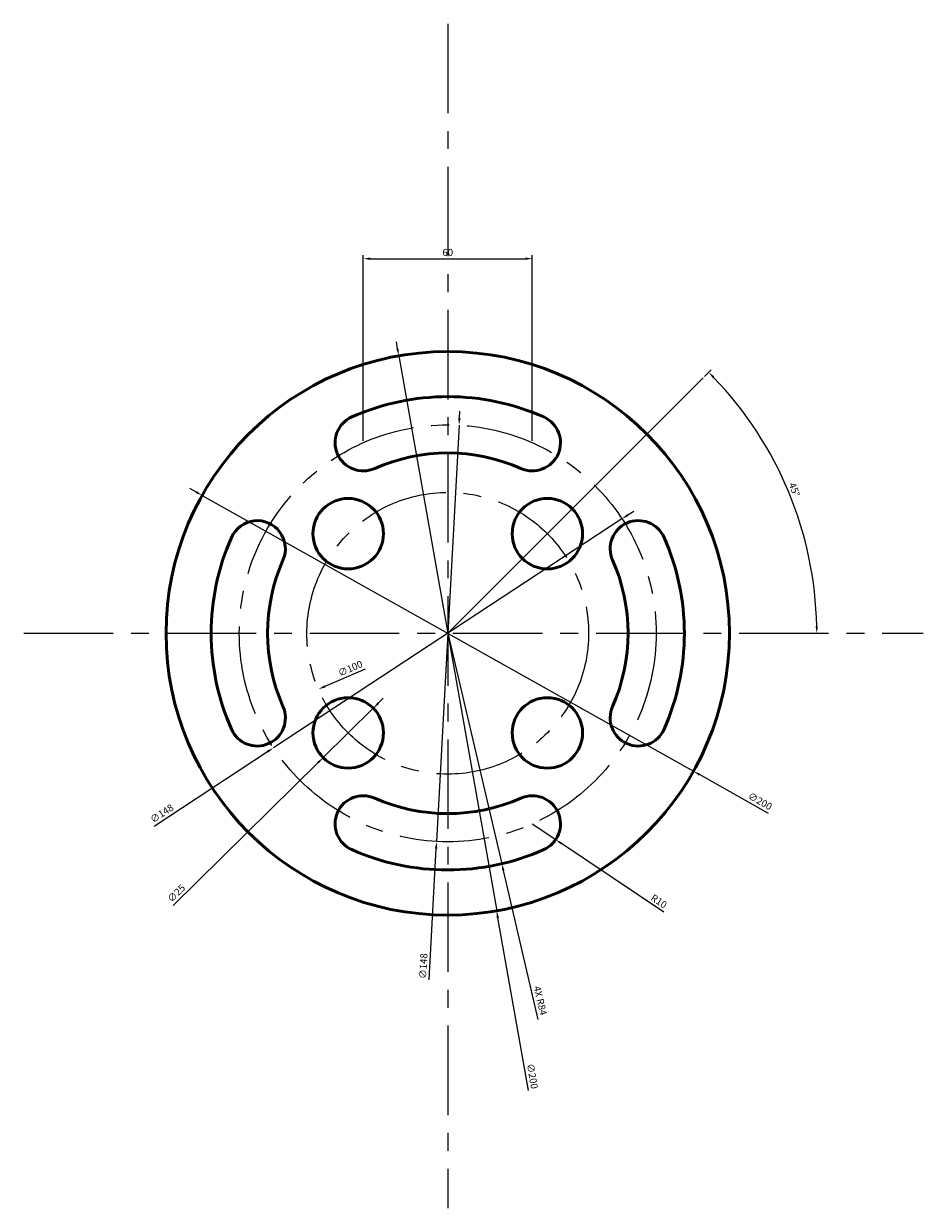
# Model space of a CAD drawing. Units: millimetres. Extents: x 2597 to 2917, y 1430 to 1850.
import ezdxf

# ---------------------------------------------------------------- set-up
doc = ezdxf.new("R2010")
doc.units = ezdxf.units.MM
doc.linetypes.add('CENTER', pattern=[50.8, 31.75, -6.35, 6.35, -6.35])
for name, color, linetype, lineweight in [('M-CNTR', 4, 'CENTER', 18), ('M-CONS', 8, 'Continuous', 18), ('M-DIMS', 2, 'Continuous', 25), ('M-OUTL', 7, 'Continuous', 50)]:
    doc.layers.add(name, color=color, linetype=linetype, lineweight=lineweight)
doc.styles.get("Standard").update_dxf_attribs({"font": 'arial.ttf'})
doc.dimstyles.new('ISO-25', dxfattribs={"dimtxt": 2.5, "dimasz": 2.5, "dimexe": 1.25, "dimexo": 0.625, "dimtad": 1, "dimdec": 1, "dimdsep": 46, "dimtxsty": 'Standard', "dimcen": 2.5, "dimadec": 0, "dimazin": 0, "dimtfac": 1, "dimtdec": 1, "dimtmove": 0, "dimatfit": 3, "dimfxl": 1, "dimarcsym": 0})

# ---------------------------------------------------------------- blocks, each defined once
blk = doc.blocks.new('*U1')
blk.add_circle((0, 0), 12.5)
blk = doc.blocks.new('*U2')
at = {"layer": 'M-OUTL', "color": 0, "linetype": 'ByBlock', "lineweight": -2, "transparency": 16777216}
for p, rotation in [((2712.64, 1669.09), 90.00000000000003), ((2712.64, 1598.38), 180), ((2783.35, 1598.38), 270)]:
    blk.add_blockref('*U1', p, dxfattribs=dict(at, rotation=rotation))
blk.add_blockref('*U1', (2783.35, 1669.09), dxfattribs=at)
blk = doc.blocks.new('*D3')
at = {"layer": 'Defpoints', "color": 0, "lineweight": 100, "transparency": 16777216}
for p in [(2777.99, 1766.69), (2717.99, 1701.38), (2777.99, 1701.38)]:
    blk.add_point(p, dxfattribs=at)
at = {"layer": 'M-DIMS', "color": 0, "lineweight": -2, "transparency": 16777216}
for p, q in [((2717.99, 1702), (2717.99, 1767.94)), ((2720.49, 1766.69), (2775.49, 1766.69)), ((2777.99, 1702), (2777.99, 1767.94))]:
    blk.add_line(p, q, dxfattribs=at)
at = {"layer": 'M-DIMS', "color": 0, "lineweight": 100, "transparency": 16777216}
for points in [[(2720.49, 1767.11), (2720.49, 1766.27), (2717.99, 1766.69)], [(2775.49, 1767.11), (2775.49, 1766.27), (2777.99, 1766.69)]]:
    blk.add_solid(points, dxfattribs=at)
at = {"layer": 'M-DIMS', "color": 0, "transparency": 16777216, "insert": (2747.99, 1768.59), "char_height": 2.5, "attachment_point": 5}
blk.add_mtext('60', dxfattribs=at)
blk = doc.blocks.new('*D4')
at = {"layer": 'Defpoints', "color": 0, "lineweight": 100, "transparency": 16777216}
for p in [(2838.63, 1724.37), (2874.53, 1667.64), (2597.44, 1633.73), (2747.99, 1633.73), (2916.81, 1633.73)]:
    blk.add_point(p, dxfattribs=at)
at = {"layer": 'M-DIMS', "color": 0, "lineweight": -2, "transparency": 16777216}
blk.add_line((2839.08, 1724.82), (2841.51, 1727.24), dxfattribs=at)
blk.add_arc((2747.99, 1633.73), 131, 1.0935, 43.9065, dxfattribs=at)
at = {"layer": 'M-DIMS', "color": 0, "lineweight": 100, "transparency": 16777216}
for points in [[(2842.08, 1724.28), (2842.67, 1724.87), (2840.62, 1726.36)], [(2879.38, 1636.24), (2878.55, 1636.23), (2878.99, 1633.73)]]:
    blk.add_solid(points, dxfattribs=at)
at = {"layer": 'M-DIMS', "color": 0, "transparency": 16777216, "insert": (2870.77, 1684.59), "char_height": 2.5, "attachment_point": 5, "rotation": 292.5}
blk.add_mtext('45°', dxfattribs=at)
blk = doc.blocks.new('*D5')
at = {"layer": 'Defpoints', "color": 0, "lineweight": 100, "transparency": 16777216}
for p in [(2793.89, 1653.58), (2702.1, 1613.89)]:
    blk.add_point(p, dxfattribs=at)
at = {"layer": 'M-DIMS', "color": 0, "lineweight": -2, "transparency": 16777216}
blk.add_line((2718.65, 1621.04), (2704.4, 1614.88), dxfattribs=at)
at = {"layer": 'M-DIMS', "color": 0, "lineweight": 100, "transparency": 16777216}
blk.add_solid([(2704.23, 1615.26), (2704.56, 1614.5), (2702.1, 1613.89)], dxfattribs=at)
at = {"layer": 'M-DIMS', "color": 0, "transparency": 16777216, "insert": (2713.51, 1620.97), "char_height": 2.5, "attachment_point": 5, "rotation": 23.3868}
blk.add_mtext('∅100', dxfattribs=at)
blk = doc.blocks.new('*D6')
at = {"layer": 'Defpoints', "color": 0, "lineweight": 100, "transparency": 16777216}
for p in [(2777.99, 1566.09), (2786.3, 1560.52)]:
    blk.add_point(p, dxfattribs=at)
at = {"layer": 'M-DIMS', "color": 0, "lineweight": -2, "transparency": 16777216}
for p, q in [((2777.99, 1566.09), (2786.3, 1560.52)), ((2824.71, 1534.76), (2788.38, 1559.12))]:
    blk.add_line(p, q, dxfattribs=at)
at = {"layer": 'M-DIMS', "color": 0, "lineweight": 100, "transparency": 16777216}
blk.add_solid([(2788.61, 1559.47), (2788.14, 1558.78), (2786.3, 1560.52)], dxfattribs=at)
at = {"layer": 'M-DIMS', "color": 0, "transparency": 16777216, "insert": (2822.77, 1538.35), "char_height": 2.5, "attachment_point": 5, "rotation": 326.1587}
blk.add_mtext('R10', dxfattribs=at)
blk = doc.blocks.new('*D7')
at = {"layer": 'Defpoints', "color": 0, "lineweight": 100, "transparency": 16777216}
for p in [(2660.79, 1682.67), (2835.2, 1584.79)]:
    blk.add_point(p, dxfattribs=at)
at = {"layer": 'M-DIMS', "color": 0, "lineweight": -2, "transparency": 16777216}
for p, q in [((2658.61, 1683.9), (2656.43, 1685.12)), ((2660.79, 1682.67), (2835.2, 1584.79)), ((2861.87, 1569.82), (2837.38, 1583.57))]:
    blk.add_line(p, q, dxfattribs=at)
at = {"layer": 'M-DIMS', "color": 0, "lineweight": 100, "transparency": 16777216}
for points in [[(2658.81, 1684.26), (2658.4, 1683.53), (2660.79, 1682.67)], [(2837.58, 1583.93), (2837.17, 1583.2), (2835.2, 1584.79)]]:
    blk.add_solid(points, dxfattribs=at)
at = {"layer": 'M-DIMS', "color": 0, "transparency": 16777216, "insert": (2858.7, 1573.86), "char_height": 2.5, "attachment_point": 5, "rotation": 330.6985}
blk.add_mtext('∅200', dxfattribs=at)
blk = doc.blocks.new('*D8')
at = {"layer": 'Defpoints', "color": 0, "lineweight": 100, "transparency": 16777216}
for p in [(2809.84, 1674.36), (2686.14, 1593.11)]:
    blk.add_point(p, dxfattribs=at)
at = {"layer": 'M-DIMS', "color": 0, "lineweight": -2, "transparency": 16777216}
for p, q in [((2809.84, 1674.36), (2686.14, 1593.11)), ((2811.93, 1675.73), (2814.02, 1677.1)), ((2643.76, 1565.27), (2684.05, 1591.73))]:
    blk.add_line(p, q, dxfattribs=at)
at = {"layer": 'M-DIMS', "color": 0, "lineweight": 100, "transparency": 16777216}
for points in [[(2811.7, 1676.08), (2812.16, 1675.38), (2809.84, 1674.36)], [(2683.82, 1592.08), (2684.28, 1591.39), (2686.14, 1593.11)]]:
    blk.add_solid(points, dxfattribs=at)
at = {"layer": 'M-DIMS', "color": 0, "transparency": 16777216, "insert": (2646.65, 1569.52), "char_height": 2.5, "attachment_point": 5, "rotation": 33.2985}
blk.add_mtext('∅148', dxfattribs=at)
blk = doc.blocks.new('*D9')
at = {"layer": 'Defpoints', "color": 0, "lineweight": 100, "transparency": 16777216}
for p in [(2721.54, 1607.15), (2703.73, 1589.6)]:
    blk.add_point(p, dxfattribs=at)
at = {"layer": 'M-DIMS', "color": 0, "lineweight": -2, "transparency": 16777216}
for p, q in [((2723.32, 1608.91), (2725.1, 1610.66)), ((2721.54, 1607.15), (2703.73, 1589.6)), ((2650.53, 1537.16), (2701.95, 1587.85))]:
    blk.add_line(p, q, dxfattribs=at)
at = {"layer": 'M-DIMS', "color": 0, "lineweight": 100, "transparency": 16777216}
for points in [[(2723.03, 1609.2), (2723.61, 1608.61), (2721.54, 1607.15)], [(2701.66, 1588.14), (2702.25, 1587.55), (2703.73, 1589.6)]]:
    blk.add_solid(points, dxfattribs=at)
at = {"layer": 'M-DIMS', "color": 0, "transparency": 16777216, "insert": (2651.84, 1541.22), "char_height": 2.5, "attachment_point": 5, "rotation": 44.5839}
blk.add_mtext('∅25', dxfattribs=at)
blk = doc.blocks.new('CURVED-SLOT-R10-PCD148')
for centre, radius, start, end in [((40, -57.65), 84, 66.0835, 113.9165), ((10, 10), 10, 113.9165, 293.9165), ((70, 10), 10, 246.0835, 66.0835), ((40, -57.65), 64, 66.0835, 113.9165)]:
    blk.add_arc(centre, radius, start, end)
blk = doc.blocks.new('*D11')
at = {"layer": 'Defpoints', "color": 0, "lineweight": 100, "transparency": 16777216}
for p in [(2730.63, 1732.21), (2765.36, 1535.25)]:
    blk.add_point(p, dxfattribs=at)
at = {"layer": 'M-DIMS', "color": 0, "lineweight": -2, "transparency": 16777216}
for p, q in [((2730.19, 1734.67), (2729.76, 1737.14)), ((2730.63, 1732.21), (2765.36, 1535.25)), ((2776.6, 1471.49), (2765.79, 1532.79))]:
    blk.add_line(p, q, dxfattribs=at)
at = {"layer": 'M-DIMS', "color": 0, "lineweight": 100, "transparency": 16777216}
for points in [[(2730.6, 1734.75), (2729.78, 1734.6), (2730.63, 1732.21)], [(2766.2, 1532.86), (2765.38, 1532.72), (2765.36, 1535.25)]]:
    blk.add_solid(points, dxfattribs=at)
at = {"layer": 'M-DIMS', "color": 0, "transparency": 16777216, "insert": (2777.72, 1476.51), "char_height": 2.5, "attachment_point": 5, "rotation": 280.0011}
blk.add_mtext('∅200', dxfattribs=at)
blk = doc.blocks.new('*D12')
at = {"layer": 'Defpoints', "color": 0, "lineweight": 100, "transparency": 16777216}
for p in [(2751.99, 1707.62), (2744, 1559.84)]:
    blk.add_point(p, dxfattribs=at)
at = {"layer": 'M-DIMS', "color": 0, "lineweight": -2, "transparency": 16777216}
for p, q in [((2752.12, 1710.12), (2752.26, 1712.62)), ((2751.99, 1707.62), (2744, 1559.84)), ((2741.35, 1510.76), (2743.87, 1557.34))]:
    blk.add_line(p, q, dxfattribs=at)
at = {"layer": 'M-DIMS', "color": 0, "lineweight": 100, "transparency": 16777216}
for points in [[(2751.71, 1710.14), (2752.54, 1710.1), (2751.99, 1707.62)], [(2743.45, 1557.37), (2744.28, 1557.32), (2744, 1559.84)]]:
    blk.add_solid(points, dxfattribs=at)
at = {"layer": 'M-DIMS', "color": 0, "transparency": 16777216, "insert": (2739.64, 1515.61), "char_height": 2.5, "attachment_point": 5, "rotation": 86.9068}
blk.add_mtext('∅148', dxfattribs=at)
blk = doc.blocks.new('*D13')
at = {"layer": 'Defpoints', "color": 0, "lineweight": 100, "transparency": 16777216}
for p in [(2747.99, 1633.73), (2767.17, 1551.95)]:
    blk.add_point(p, dxfattribs=at)
at = {"layer": 'M-DIMS', "color": 0, "lineweight": -2, "transparency": 16777216}
for p, q in [((2747.99, 1633.73), (2767.17, 1551.95)), ((2780.12, 1496.71), (2767.74, 1549.52))]:
    blk.add_line(p, q, dxfattribs=at)
at = {"layer": 'M-DIMS', "color": 0, "lineweight": 100, "transparency": 16777216}
blk.add_solid([(2768.15, 1549.61), (2767.33, 1549.42), (2767.17, 1551.95)], dxfattribs=at)
at = {"layer": 'M-DIMS', "color": 0, "transparency": 16777216, "insert": (2780.53, 1503.32), "char_height": 2.5, "attachment_point": 5, "rotation": 283.1967}
blk.add_mtext('4X R84', dxfattribs=at)

msp = doc.modelspace()

# ---------------------------------------------------------------- linework, layer by layer
at = {"layer": 'M-CNTR'}
for p, q in [((2747.99, 1850.09), (2747.99, 1429.65)), ((2597.44, 1633.73), (2916.81, 1633.73))]:
    msp.add_line(p, q, dxfattribs=at)
for radius in [74, 50]:
    msp.add_circle((2747.99, 1633.73), radius, dxfattribs=at)
at = {"layer": 'M-CONS'}
msp.add_line((2747.99, 1633.73), (2838.63, 1724.37), dxfattribs=at)
at = {"layer": 'M-OUTL'}
msp.add_circle((2747.99, 1633.73), 100, dxfattribs=at)

# ---------------------------------------------------------------- block references
for name, p in [('CURVED-SLOT-R10-PCD148', (2707.99, 1691.38)), ('*U2', (0, 0))]:
    msp.add_blockref(name, p, dxfattribs=at)
for p, rotation in [((2690.35, 1593.73), 89.99999999999909), ((2805.64, 1673.73), 269.9999999999991), ((2787.99, 1576.09), 180)]:
    msp.add_blockref('CURVED-SLOT-R10-PCD148', p, dxfattribs=dict(at, rotation=rotation))

# ---------------------------------------------------------------- dimensions: what is measured, and where the dimension line sits
at = {"layer": 'M-DIMS'}
dim = msp.add_aligned_dim(p1=(2717.99, 1701.38), p2=(2777.99, 1701.38), distance=65.31, dimstyle='ISO-25', override={"dimclrd": 0, "dimclre": 0, "dimclrt": 0}, dxfattribs=at)
dim.commit()
dim.dimension.update_dxf_attribs({"geometry": '*D3', "text_midpoint": (2747.99, 1768.59)})
for p1, p2, override, picture, middle in [((2730.63, 1732.21), (2765.36, 1535.25), {"dimdec": 0, "dimlfac": 1, "dimrnd": 0, "dimzin": 0, "dimdsep": 46, "dimlunit": 2}, '*D11', (2775.78, 1476.16)), ((2751.99, 1707.62), (2744, 1559.84), {"dimdec": 0, "dimlfac": 1, "dimrnd": 0, "dimzin": 0, "dimdsep": 46, "dimlunit": 2}, '*D12', (2741.6, 1515.5)), ((2660.79, 1682.67), (2835.2, 1584.79), {"dimclrd": 0, "dimclre": 0, "dimclrt": 0}, '*D7', (2857.73, 1572.14)), ((2809.84, 1674.36), (2686.14, 1593.11), {"dimclrd": 0, "dimclre": 0, "dimclrt": 0}, '*D8', (2647.73, 1567.88)), ((2793.89, 1653.58), (2702.1, 1613.89), {"dimclrd": 0, "dimclre": 0, "dimclrt": 0}, '*D5', (2714.29, 1619.16)), ((2721.54, 1607.15), (2703.73, 1589.6), {"dimclrd": 0, "dimclre": 0, "dimclrt": 0}, '*D9', (2653.22, 1539.82))]:
    dim = msp.add_diameter_dim_2p(p1=p1, p2=p2, dimstyle='ISO-25', override=override, dxfattribs=at)
    dim.commit()
    dim.dimension.update_dxf_attribs({"geometry": picture, "text_midpoint": middle, "dimtype": 163})
dim = msp.add_angular_dim_2l(base=(2874.53, 1667.64), line1=((2597.44, 1633.73), (2916.81, 1633.73)), line2=((2747.99, 1633.73), (2838.63, 1724.37)), dimstyle='ISO-25', override={"dimclrd": 0, "dimclre": 0, "dimclrt": 0}, dxfattribs=at)
dim.commit()
dim.dimension.update_dxf_attribs({"geometry": '*D4', "text_midpoint": (2870.77, 1684.59)})
dim = msp.add_radius_dim(center=(2747.99, 1633.73), mpoint=(2767.17, 1551.95), text='4X <>', dimstyle='ISO-25', override={"dimdec": 0, "dimlfac": 1, "dimrnd": 0, "dimzin": 0, "dimdsep": 46, "dimlunit": 2}, dxfattribs=at)
dim.commit()
dim.dimension.update_dxf_attribs({"geometry": '*D13', "text_midpoint": (2778.68, 1502.88), "dimtype": 164})
dim = msp.add_radius_dim(center=(2777.99, 1566.09), mpoint=(2786.3, 1560.52), dimstyle='ISO-25', override={"dimclrd": 0, "dimclre": 0, "dimclrt": 0}, dxfattribs=at)
dim.commit()
dim.dimension.update_dxf_attribs({"geometry": '*D6', "text_midpoint": (2821.72, 1536.77), "dimtype": 164})

doc.saveas('drawing.dxf')
